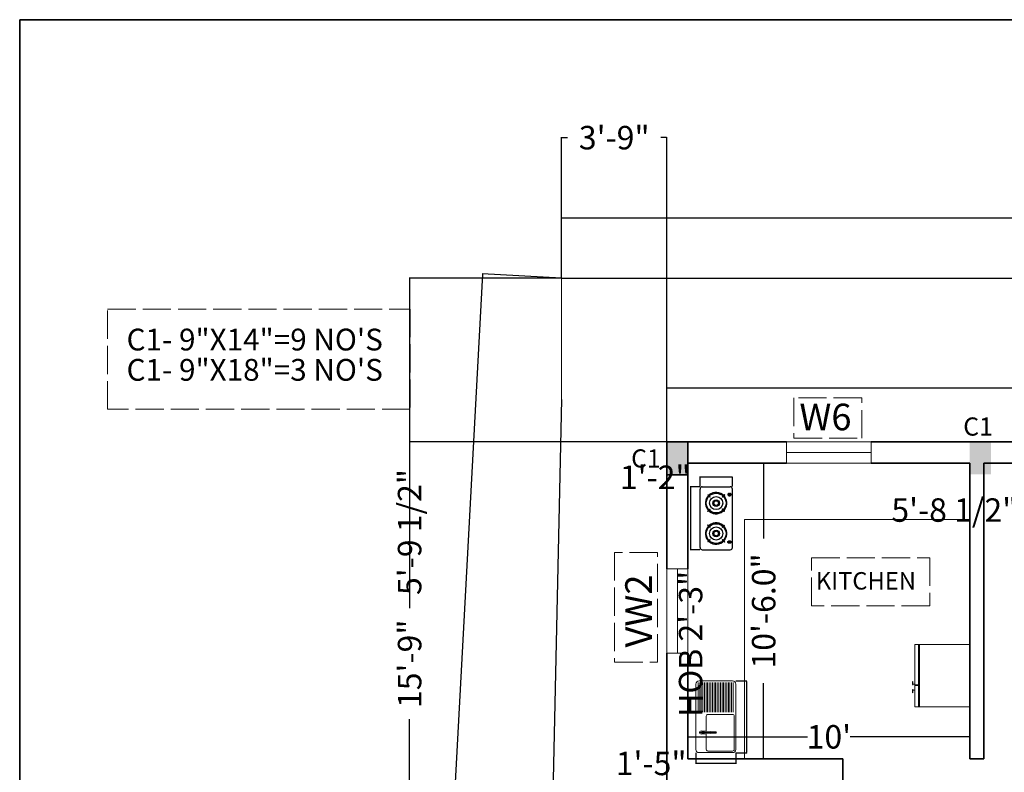
# Model space of a CAD drawing. Units: inches. Extents: x -269 to 4574, y -694 to 313.
# Tile 9 of 19: x -269 to 151, y -122 to 198. Entities that reach past the tile are written whole.
import ezdxf

# ---------------------------------------------------------------- set-up
doc = ezdxf.new("R2010")
doc.units = ezdxf.units.IN
doc.header["$MEASUREMENT"] = 0
doc.linetypes.add('ACAD_ISO02W100', pattern=[15, 12, -3])
for name, color, linetype, lineweight in [('A-ANNO-FRAM', 7, 'ACAD_ISO02W100', 13), ('A-ANNO-IDEN', 6, 'Continuous', 18), ('A-AREA-IDEN', 6, 'Continuous', 20), ('A-COLS', 5, 'Continuous', 35), ('A-COLS-IDEN', 6, 'Continuous', 18), ('A-COLS-PATT', 5, 'Continuous', 35), ('A-EQPM', 21, 'Continuous', 18), ('A-FLOR-CASE', 2, 'Continuous', 18), ('A-FLOR-FIXT', 21, 'Continuous', 18), ('BORDER', 7, 'Continuous', 35), ('C-PROP', 7, 'Continuous', 25), ('DIMENSION', 5, 'Continuous', 18), ('WALL', 1, 'Continuous', 35), ('WINDOWS', 2, 'Continuous', 18)]:
    doc.layers.add(name, color=color, linetype=linetype, lineweight=lineweight)
doc.layers.add('NOI THAT', color=42, linetype='Continuous')
doc.dimstyles.get("Standard").update_dxf_attribs({"dimtxt": 10, "dimasz": 0.18, "dimexe": 0.18, "dimexo": 0.0625, "dimgap": 0.09, "dimtad": 0, "dimdec": 1, "dimzin": 0, "dimdsep": 46, "dimlunit": 3, "dimtxsty": 'Standard', "dimcen": 0.09, "dimclrt": 7, "dimadec": 0, "dimazin": 0, "dimtfac": 1, "dimtdec": 1, "dimtofl": 0, "dimtmove": 0, "dimatfit": 3, "dimfxl": 1, "dimtolj": 1, "dimtzin": 0, "dimarcsym": 0})

# ---------------------------------------------------------------- blocks, each defined once
blk = doc.blocks.new('*D1')
at = {"layer": 'Defpoints', "color": 0, "lineweight": 0, "transparency": 16777216}
for p in [(451.14, 41.26), (7.14, 18.27), (451.14, 18.27)]:
    blk.add_point(p, dxfattribs=at)
at = {"layer": 'DIMENSION', "color": 0, "lineweight": -2, "transparency": 16777216}
for p, q in [((7.14, 18.33), (7.14, 41.44)), ((7.32, 41.26), (219.05, 41.26)), ((450.96, 41.26), (239.23, 41.26)), ((451.14, 18.33), (451.14, 41.44))]:
    blk.add_line(p, q, dxfattribs=at)
at = {"layer": 'DIMENSION', "color": 0, "lineweight": 0, "transparency": 16777216}
for points in [[(7.32, 41.29), (7.32, 41.23), (7.14, 41.26)], [(450.96, 41.29), (450.96, 41.23), (451.14, 41.26)]]:
    blk.add_solid(points, dxfattribs=at)
at = {"layer": 'DIMENSION', "color": 0, "transparency": 16777216, "insert": (229.14, 41.26), "char_height": 10, "attachment_point": 5}
blk.add_mtext("\\A1;37'", dxfattribs=at)
blk = doc.blocks.new('SINK90X50')
for p, q in [((-57, 553), (-430, 553)), ((-57, 533), (-430, 533)), ((-57, 513), (-430, 513)), ((192, 455), (177, 516)), ((187, 334), (177, 516)), ((197, 536), (197, 324)), ((202, 455), (217, 516)), ((207, 334), (217, 516)), ((-57, 493), (-430, 493)), ((-57, 473), (-430, 473)), ((-57, 453), (-430, 453)), ((-57, 433), (-430, 433)), ((-57, 413), (-430, 413)), ((-57, 393), (-430, 393)), ((-57, 373), (-430, 373)), ((-57, 353), (-430, 353)), ((-57, 333), (-430, 333)), ((-57, 313), (-430, 313)), ((-57, 293), (-430, 293)), ((-57, 273), (-430, 273)), ((-57, 253), (-430, 253)), ((-57, 233), (-430, 233)), ((-57, 213), (-430, 213)), ((-57, 193), (-430, 193)), ((-57, 173), (-430, 173)), ((-57, 153), (-430, 153)), ((-57, 133), (-430, 133)), ((-57, 113), (-430, 113))]:
    blk.add_line(p, q)
blk.add_lwpolyline([(450, 540, 0.414214), (410, 580), (-410, 580, 0.414214), (-450, 540), (-450, 120, 0.414214), (-410, 80), (410, 80, 0.414214), (450, 120)], format="xyb", close=True)
blk.add_lwpolyline([(181, 450), (-10, 450, 0.414214), (-30, 430), (-30, 120, 0.414214), (-10, 100), (410, 100, 0.414214), (430, 120), (430, 430, 0.414214), (410, 450), (214, 450)], format="xyb")
for centre, radius, start, end in [((197, 516), 20, 351.3062, 188.6938), ((197, 455), 5, 180, 0), ((197, 334), 10, 180, 0)]:
    blk.add_arc(centre, radius, start, end)
for points in [[(187, 506), (181, 513), (189, 496), (197, 479)], [(207, 506), (214, 513), (206, 496), (197, 479)]]:
    blk.add_open_spline(points, degree=3)
blk = doc.blocks.new('A$C2C6C0730')
at = {"layer": 'NOI THAT'}
for p, q in [((0, 1353), (0, 50)), ((670, 1403), (50, 1403)), ((720, 1353), (720, 50)), ((670, 0), (50, 0))]:
    blk.add_line(p, q, dxfattribs=at)
for points in [[(66, 1257, -0.070182), (81, 1254, -0.081942), (93, 1249, -0.106897), (102, 1239, -0.135195), (105, 1230, -0.135195), (102, 1220, -0.106897), (93, 1210, -0.081942), (81, 1205, -0.070182), (66, 1203, -0.070182), (50, 1205, -0.081942), (38, 1210, -0.106897), (30, 1220, -0.135195), (27, 1230, -0.135195), (30, 1239, -0.106897), (38, 1249, -0.081942), (50, 1254, -0.070182)], [(66, 146, 0.070182), (81, 148, 0.081942), (93, 154, 0.106897), (102, 163, 0.135195), (105, 173, 0.135195), (102, 183, 0.106897), (93, 192, 0.081942), (81, 198, 0.070182), (66, 200, 0.070182), (50, 198, 0.081942), (38, 192, 0.106897), (30, 183, 0.135195), (27, 173, 0.135195), (30, 163, 0.106897), (38, 154, 0.081942), (50, 148, 0.070182)]]:
    blk.add_lwpolyline(points, format="xyb", close=True, dxfattribs=at)
for points in [[(68, 1203), (68, 1257), (62, 1257), (62, 1203)], [(220, 1175), (171, 1223), (179, 1230), (227, 1182)], [(541, 1226), (493, 1177), (500, 1170), (548, 1219)], [(176, 861), (224, 909), (232, 902), (183, 853)], [(497, 897), (546, 849), (553, 856), (505, 904)], [(176, 542), (224, 494), (232, 501), (183, 550)], [(497, 506), (546, 554), (553, 547), (505, 498)], [(220, 228), (171, 180), (179, 172), (227, 221)], [(541, 177), (493, 225), (500, 233), (548, 184)], [(68, 200), (68, 146), (62, 146), (62, 200)]]:
    blk.add_lwpolyline(points, close=True, dxfattribs=at)
for centre, radius in [((362, 1040), 219), ((362, 1040), 145), ((362, 1040), 72.6), ((362, 1040), 51.5), ((362, 363), 219), ((362, 363), 145), ((362, 363), 72.6), ((362, 363), 51.5)]:
    blk.add_circle(centre, radius, dxfattribs=at)
for centre, radius, start, end in [((50, 1353), 50, 90, 180), ((670, 1353), 50, 0, 90), ((65, 1230), 19.4, 99.7177, 260.2823), ((65, 1230), 19.4, 279.9102, 80.0898), ((362, 1040), 238, 152.4796, 149.9329), ((362, 363), 238, 210.0671, 207.5204), ((50, 50), 50, 180, 270), ((65, 173), 19.4, 99.7177, 260.2823), ((65, 173), 19.4, 279.9102, 80.0898), ((670, 50), 50, 270, 0)]:
    blk.add_arc(centre, radius, start, end, dxfattribs=at)
blk = doc.blocks.new('*D16')
at = {"layer": 'Defpoints', "color": 0, "lineweight": 0, "transparency": 16777216}
for p in [(16.14, -107.35), (16.14, -116.73), (136.14, -116.73)]:
    blk.add_point(p, dxfattribs=at)
at = {"layer": 'DIMENSION', "color": 0, "lineweight": -2, "transparency": 16777216}
for p, q in [((16.14, -116.67), (16.14, -107.17)), ((16.32, -107.35), (67, -107.35)), ((135.96, -107.35), (85.27, -107.35)), ((136.14, -116.67), (136.14, -107.17))]:
    blk.add_line(p, q, dxfattribs=at)
at = {"layer": 'DIMENSION', "color": 0, "lineweight": 0, "transparency": 16777216}
for points in [[(16.32, -107.32), (16.32, -107.38), (16.14, -107.35)], [(135.96, -107.32), (135.96, -107.38), (136.14, -107.35)]]:
    blk.add_solid(points, dxfattribs=at)
at = {"layer": 'DIMENSION', "color": 0, "transparency": 16777216, "insert": (76.14, -107.35), "char_height": 10, "attachment_point": 5}
blk.add_mtext("\\A1;10'", dxfattribs=at)
blk = doc.blocks.new('*D17')
at = {"layer": 'Defpoints', "color": 0, "lineweight": 0, "transparency": 16777216}
for p in [(40.14, 9.27), (48.37, 9.27), (40.14, -116.73)]:
    blk.add_point(p, dxfattribs=at)
at = {"layer": 'DIMENSION', "color": 0, "lineweight": -2, "transparency": 16777216}
for p, q in [((40.2, 9.27), (48.55, 9.27)), ((48.37, 9.09), (48.37, -22.93)), ((48.37, -116.55), (48.37, -84.54)), ((40.2, -116.73), (48.55, -116.73))]:
    blk.add_line(p, q, dxfattribs=at)
at = {"layer": 'DIMENSION', "color": 0, "lineweight": 0, "transparency": 16777216}
for points in [[(48.34, 9.09), (48.4, 9.09), (48.37, 9.27)], [(48.34, -116.55), (48.4, -116.55), (48.37, -116.73)]]:
    blk.add_solid(points, dxfattribs=at)
at = {"layer": 'DIMENSION', "color": 0, "transparency": 16777216, "insert": (48.37, -53.73), "char_height": 10, "attachment_point": 5, "rotation": 90}
blk.add_mtext('\\A1;10\'-6.0"', dxfattribs=at)
blk = doc.blocks.new('*D32')
at = {"layer": 'Defpoints', "color": 0, "lineweight": 0, "transparency": 16777216}
for p in [(-37.71, 113.85), (478.29, 113.67), (478.29, 113.64)]:
    blk.add_point(p, dxfattribs=at)
at = {"layer": 'DIMENSION', "color": 0, "lineweight": -2, "transparency": 16777216}
for p, q in [((-37.71, 113.79), (-37.71, 113.46)), ((-37.53, 113.64), (210.2, 113.64)), ((478.11, 113.64), (230.38, 113.64)), ((478.29, 113.61), (478.29, 113.46))]:
    blk.add_line(p, q, dxfattribs=at)
at = {"layer": 'DIMENSION', "color": 0, "lineweight": 0, "transparency": 16777216}
for points in [[(-37.53, 113.67), (-37.53, 113.61), (-37.71, 113.64)], [(478.11, 113.67), (478.11, 113.61), (478.29, 113.64)]]:
    blk.add_solid(points, dxfattribs=at)
at = {"layer": 'DIMENSION', "color": 0, "transparency": 16777216, "insert": (220.29, 113.64), "char_height": 10, "attachment_point": 5}
blk.add_mtext("\\A1;43'", dxfattribs=at)
blk = doc.blocks.new('*D34')
at = {"layer": 'Defpoints', "color": 0, "lineweight": 0, "transparency": 16777216}
for p in [(-37.71, 88), (-102.08, -478.85), (-68.45, -480.67)]:
    blk.add_point(p, dxfattribs=at)
at = {"layer": 'DIMENSION', "color": 0, "lineweight": -2, "transparency": 16777216}
for p, q in [((-71.35, 89.64), (-85, -162.81)), ((-37.77, 88), (-71.52, 89.83)), ((-102.07, -478.67), (-88.43, -226.23)), ((-68.51, -480.67), (-102.26, -478.84))]:
    blk.add_line(p, q, dxfattribs=at)
at = {"layer": 'DIMENSION', "color": 0, "lineweight": 0, "transparency": 16777216}
for points in [[(-71.38, 89.64), (-71.32, 89.64), (-71.34, 89.82)], [(-102.1, -478.67), (-102.04, -478.67), (-102.08, -478.85)]]:
    blk.add_solid(points, dxfattribs=at)
at = {"layer": 'DIMENSION', "color": 0, "transparency": 16777216, "insert": (-86.71, -194.52), "char_height": 10, "attachment_point": 5, "rotation": 86.9054}
blk.add_mtext('\\A1;47\'-5.5"', dxfattribs=at)
blk = doc.blocks.new('GLAZ-36IN')
blk.add_line((0, 4.5), (36, 4.5))
blk.add_lwpolyline([(0, 9), (36, 9), (36, 0), (0, 0)], close=True)
blk = doc.blocks.new('COLUMN-9x14-PLAN')
h = blk.add_hatch(color=256)
h.dxf.hatch_style = 1
h.paths.add_polyline_path([(9, 14), (0, 14), (0, 0), (9, 0), (9, 5)])
blk = doc.blocks.new('*D61')
at = {"layer": 'Defpoints', "color": 0, "lineweight": 0, "transparency": 16777216}
for p in [(36.5, -83.55), (36.5, -114.1), (41.08, -114.1)]:
    blk.add_point(p, dxfattribs=at)
at = {"layer": 'DIMENSION', "color": 0, "lineweight": -2, "transparency": 16777216}
for p, q in [((36.56, -83.55), (41.26, -83.55)), ((41.08, -83.73), (41.08, -113.92)), ((36.56, -114.1), (41.26, -114.1)), ((41.08, -114.1), (41.08, -114.28))]:
    blk.add_line(p, q, dxfattribs=at)
at = {"layer": 'DIMENSION', "color": 0, "lineweight": 0, "transparency": 16777216}
for points in [[(41.05, -83.73), (41.11, -83.73), (41.08, -83.55)], [(41.05, -113.92), (41.11, -113.92), (41.08, -114.1)]]:
    blk.add_solid(points, dxfattribs=at)
at = {"layer": 'DIMENSION', "color": 7, "transparency": 16777216, "insert": (41.08, -173.89), "char_height": 10, "attachment_point": 5, "rotation": 90}
blk.add_mtext('\\A1;SINK 2\'-6 1/2"', dxfattribs=at)
blk = doc.blocks.new('*D62')
at = {"layer": 'Defpoints', "color": 0, "lineweight": 0, "transparency": 16777216}
for p in [(19.53, -114.1), (36.5, -114.1), (19.53, -118.68)]:
    blk.add_point(p, dxfattribs=at)
at = {"layer": 'DIMENSION', "color": 0, "lineweight": -2, "transparency": 16777216}
for p, q in [((19.53, -114.16), (19.53, -118.86)), ((36.5, -114.16), (36.5, -118.86)), ((19.53, -118.68), (19.35, -118.68)), ((36.32, -118.68), (19.71, -118.68))]:
    blk.add_line(p, q, dxfattribs=at)
at = {"layer": 'DIMENSION', "color": 0, "lineweight": 0, "transparency": 16777216}
for points in [[(19.71, -118.65), (19.71, -118.71), (19.53, -118.68)], [(36.32, -118.65), (36.32, -118.71), (36.5, -118.68)]]:
    blk.add_solid(points, dxfattribs=at)
at = {"layer": 'DIMENSION', "color": 7, "transparency": 16777216, "insert": (0.45, -118.68), "char_height": 10, "attachment_point": 5}
blk.add_mtext('\\A1;1\'-5"', dxfattribs=at)
blk = doc.blocks.new('*D63')
at = {"layer": 'Defpoints', "color": 0, "lineweight": 0, "transparency": 16777216}
for p in [(21.28, -0.84), (17.25, -27.7), (21.28, -27.7)]:
    blk.add_point(p, dxfattribs=at)
at = {"layer": 'DIMENSION', "color": 0, "lineweight": -2, "transparency": 16777216}
for p, q in [((21.22, -0.84), (17.07, -0.84)), ((17.25, -1.02), (17.25, -27.52)), ((21.22, -27.7), (17.07, -27.7)), ((17.25, -27.7), (17.25, -27.88))]:
    blk.add_line(p, q, dxfattribs=at)
at = {"layer": 'DIMENSION', "color": 0, "lineweight": 0, "transparency": 16777216}
for points in [[(17.22, -1.02), (17.28, -1.02), (17.25, -0.84)], [(17.22, -27.52), (17.28, -27.52), (17.25, -27.7)]]:
    blk.add_solid(points, dxfattribs=at)
at = {"layer": 'DIMENSION', "color": 7, "transparency": 16777216, "insert": (17.25, -67.74), "char_height": 10, "attachment_point": 5, "rotation": 90}
blk.add_mtext('\\A1;HOB 2\'-3"', dxfattribs=at)
blk = doc.blocks.new('*D64')
at = {"layer": 'Defpoints', "color": 0, "lineweight": 0, "transparency": 16777216}
for p in [(21.28, 3.19), (21.28, -0.84), (35.07, -0.84)]:
    blk.add_point(p, dxfattribs=at)
at = {"layer": 'DIMENSION', "color": 0, "lineweight": -2, "transparency": 16777216}
for p, q in [((21.28, 3.19), (21.1, 3.19)), ((21.28, -0.78), (21.28, 3.37)), ((34.89, 3.19), (21.46, 3.19)), ((35.07, -0.78), (35.07, 3.37))]:
    blk.add_line(p, q, dxfattribs=at)
at = {"layer": 'DIMENSION', "color": 0, "lineweight": 0, "transparency": 16777216}
for points in [[(21.46, 3.22), (21.46, 3.16), (21.28, 3.19)], [(34.89, 3.22), (34.89, 3.16), (35.07, 3.19)]]:
    blk.add_solid(points, dxfattribs=at)
at = {"layer": 'DIMENSION', "color": 7, "transparency": 16777216, "insert": (2.2, 3.19), "char_height": 10, "attachment_point": 5}
blk.add_mtext('\\A1;1\'-2"', dxfattribs=at)
blk = doc.blocks.new('*D66')
at = {"layer": 'Defpoints', "color": 0, "lineweight": 0, "transparency": 16777216}
for p in [(167.97, -10.77), (167.97, -24.12), (236.53, -24.12)]:
    blk.add_point(p, dxfattribs=at)
at = {"layer": 'DIMENSION', "color": 0, "lineweight": -2, "transparency": 16777216}
for p, q in [((167.97, -10.77), (167.79, -10.77)), ((167.97, -24.05), (167.97, -10.59)), ((236.35, -10.77), (168.15, -10.77)), ((236.53, -24.05), (236.53, -10.59))]:
    blk.add_line(p, q, dxfattribs=at)
at = {"layer": 'DIMENSION', "color": 0, "lineweight": 0, "transparency": 16777216}
for points in [[(168.15, -10.74), (168.15, -10.8), (167.97, -10.77)], [(236.35, -10.74), (236.35, -10.8), (236.53, -10.77)]]:
    blk.add_solid(points, dxfattribs=at)
at = {"layer": 'DIMENSION', "color": 7, "transparency": 16777216, "insert": (129.6, -10.77), "char_height": 10, "attachment_point": 5}
blk.add_mtext('\\A1;5\'-8 1/2"', dxfattribs=at)
blk = doc.blocks.new('*D74')
at = {"layer": 'Defpoints', "color": 0, "lineweight": 0, "transparency": 16777216}
for p in [(-37.71, 88), (-102.45, 18.27), (7.14, 18.27)]:
    blk.add_point(p, dxfattribs=at)
at = {"layer": 'DIMENSION', "color": 0, "lineweight": -2, "transparency": 16777216}
for p, q in [((-37.77, 88), (-102.63, 88)), ((-102.45, 87.82), (-102.45, 18.45)), ((7.07, 18.27), (-102.63, 18.27)), ((-102.45, 18.27), (-102.45, 18.09))]:
    blk.add_line(p, q, dxfattribs=at)
at = {"layer": 'DIMENSION', "color": 0, "lineweight": 0, "transparency": 16777216}
for points in [[(-102.48, 87.82), (-102.42, 87.82), (-102.45, 88)], [(-102.48, 18.45), (-102.42, 18.45), (-102.45, 18.27)]]:
    blk.add_solid(points, dxfattribs=at)
at = {"layer": 'DIMENSION', "color": 7, "transparency": 16777216, "insert": (-102.45, -20.1), "char_height": 10, "attachment_point": 5, "rotation": 90}
blk.add_mtext('\\A1;5\'-9 1/2"', dxfattribs=at)
blk = doc.blocks.new('*D75')
at = {"layer": 'Defpoints', "color": 0, "lineweight": 0, "transparency": 16777216}
for p in [(7.14, 147.85), (-37.71, 88), (7.14, 18.27)]:
    blk.add_point(p, dxfattribs=at)
at = {"layer": 'DIMENSION', "color": 0, "lineweight": -2, "transparency": 16777216}
for p, q in [((-37.71, 88.06), (-37.71, 148.03)), ((-37.53, 147.85), (-35.14, 147.85)), ((6.96, 147.85), (4.57, 147.85)), ((7.14, 18.33), (7.14, 148.03))]:
    blk.add_line(p, q, dxfattribs=at)
at = {"layer": 'DIMENSION', "color": 0, "lineweight": 0, "transparency": 16777216}
for points in [[(-37.53, 147.88), (-37.53, 147.82), (-37.71, 147.85)], [(6.96, 147.88), (6.96, 147.82), (7.14, 147.85)]]:
    blk.add_solid(points, dxfattribs=at)
at = {"layer": 'DIMENSION', "color": 7, "transparency": 16777216, "insert": (-15.28, 147.85), "char_height": 10, "attachment_point": 5}
blk.add_mtext('\\A1;3\'-9"', dxfattribs=at)
blk = doc.blocks.new('*D76')
at = {"layer": 'Defpoints', "color": 0, "lineweight": 0, "transparency": 16777216}
for p in [(7.14, 18.27), (-102.45, -170.73), (16.14, -170.73)]:
    blk.add_point(p, dxfattribs=at)
at = {"layer": 'DIMENSION', "color": 0, "lineweight": -2, "transparency": 16777216}
for p, q in [((7.07, 18.27), (-102.63, 18.27)), ((-102.45, 18.09), (-102.45, -52.57)), ((-102.45, -170.55), (-102.45, -99.89)), ((16.07, -170.73), (-102.63, -170.73))]:
    blk.add_line(p, q, dxfattribs=at)
at = {"layer": 'DIMENSION', "color": 0, "lineweight": 0, "transparency": 16777216}
for points in [[(-102.48, 18.09), (-102.42, 18.09), (-102.45, 18.27)], [(-102.48, -170.55), (-102.42, -170.55), (-102.45, -170.73)]]:
    blk.add_solid(points, dxfattribs=at)
at = {"layer": 'DIMENSION', "color": 7, "transparency": 16777216, "insert": (-102.45, -76.23), "char_height": 10, "attachment_point": 5, "rotation": 90}
blk.add_mtext('\\A1;15\'-9"', dxfattribs=at)

msp = doc.modelspace()

# ---------------------------------------------------------------- hatches: boundary and pattern name
at = {"layer": 'A-COLS-PATT'}
h = msp.add_hatch(color=256, dxfattribs=at)
h.dxf.hatch_style = 1
h.paths.add_polyline_path([(16.14, 18.27), (7.14, 18.27), (7.14, 4.27), (16.14, 4.27), (16.14, 9.27)])

# ---------------------------------------------------------------- linework, layer by layer
at = {"layer": 'A-ANNO-FRAM'}
for points in [[(-231.08, 74.85), (-102.18, 74.85), (-102.18, 32.18), (-231.08, 32.18)], [(90.18, 36.98), (61.24, 36.98), (61.24, 19.84), (90.18, 19.84)], [(3.2, -28.82), (-15.16, -28.82), (-15.16, -75.62), (3.2, -75.62)], [(68.75, -31.06), (119.14, -31.06), (119.14, -51.51), (68.75, -51.51)]]:
    msp.add_lwpolyline(points, close=True, dxfattribs=at)
at = {"layer": 'A-COLS'}
for p, q in [((16.14, 9.27), (16.14, 18.27)), ((7.14, 4.27), (16.14, 4.27))]:
    msp.add_line(p, q, dxfattribs=at)
at = {"layer": 'A-EQPM'}
for points, invisible_edges in [([(112.8, -85.17, 51.35), (112.8, -85.17, 51.35), (112.8, -68.06, 3.11), (112.8, -85.17, 3.11)], 2), ([(112.8, -68.06, 3.11), (112.8, -68.06, 3.11), (112.8, -85.17, 51.35), (112.8, -68.06, 51.35)], 2), ([(114.35, -68.06, 3.11), (114.35, -68.06, 3.11), (112.8, -68.06, 51.35), (114.35, -68.06, 51.35)], 2), ([(112.8, -68.06, 51.35), (112.8, -68.06, 51.35), (114.35, -68.06, 3.11), (112.8, -68.06, 3.11)], 2), ([(112.8, -68.06, 51.35), (112.8, -68.06, 51.35), (114.35, -85.17, 51.35), (114.35, -68.06, 51.35)], 2), ([(114.35, -85.17, 51.35), (114.35, -85.17, 51.35), (112.8, -68.06, 51.35), (112.8, -85.17, 51.35)], 2), ([(114.74, -68.06), (114.74, -68.06), (136.14, -68.06, 51.35), (136.14, -68.06)], 2), ([(136.14, -68.06, 51.35), (136.14, -68.06, 51.35), (114.74, -68.06), (114.74, -68.06, 51.35)], 2), ([(114.74, -94.51, 3.11), (114.74, -94.51, 3.11), (114.74, -68.06), (114.74, -94.51)], 2), ([(114.74, -68.06), (114.74, -68.06), (114.74, -94.51, 3.11), (114.74, -68.06, 3.11)], 2), ([(114.74, -68.06, 51.35), (114.74, -68.06, 51.35), (136.14, -94.51, 51.35), (136.14, -68.06, 51.35)], 2), ([(136.14, -94.51, 51.35), (136.14, -94.51, 51.35), (114.74, -68.06, 51.35), (114.74, -94.51, 51.35)], 2), ([(136.14, -68.06, 51.35), (136.14, -68.06, 51.35), (136.14, -94.51), (136.14, -68.06)], 2), ([(136.14, -94.51), (136.14, -94.51), (136.14, -68.06, 51.35), (136.14, -94.51, 51.35)], 2), ([(112.8, -94.51, 51.35), (112.8, -94.51, 51.35), (112.8, -85.56, 3.11), (112.8, -94.51, 3.11)], 2), ([(112.8, -85.56, 3.11), (112.8, -85.56, 3.11), (112.8, -94.51, 51.35), (112.8, -85.56, 51.35)], 2), ([(114.35, -85.56, 51.35), (114.35, -85.56, 51.35), (112.8, -94.51, 51.35), (114.35, -94.51, 51.35)], 2), ([(112.8, -94.51, 51.35), (112.8, -94.51, 51.35), (114.35, -85.56, 51.35), (112.8, -85.56, 51.35)], 2), ([(114.35, -94.51, 3.11), (114.35, -94.51, 3.11), (114.35, -94.51, 51.35), (112.8, -94.51, 51.35)], 9), ([(112.8, -94.51, 51.35), (112.8, -94.51, 51.35), (112.8, -94.51, 3.11), (114.35, -94.51, 3.11)], 9), ([(114.74, -94.51), (114.74, -94.51), (136.14, -94.51), (136.14, -94.51, 51.35)], 9), ([(136.14, -94.51, 51.35), (136.14, -94.51, 51.35), (114.74, -94.51, 51.35), (114.74, -94.51)], 9)]:
    msp.add_3dface(points, dxfattribs=dict(at, invisible_edges=invisible_edges))
at = {"layer": 'A-FLOR-CASE'}
for p, q in [((40.14, -116.73), (40.14, -14.73)), ((40.14, -14.73), (136.14, -14.73))]:
    msp.add_line(p, q, dxfattribs=at)
at = {"layer": 'BORDER'}
msp.add_lwpolyline([(-268.51, 198.09), (666.62, 198.09), (666.62, -693.82), (-268.51, -693.82)], close=True, dxfattribs=at)
at = {"layer": 'C-PROP'}
for p, q in [((-37.71, 88), (478.29, 88)), ((-37.71, 36.26), (-49.71, -506.83))]:
    msp.add_line(p, q, dxfattribs=at)
at = {"layer": 'DIMENSION'}
msp.add_line((-37.71, 36.32), (-37.71, 113.85), dxfattribs=at)
msp.add_solid([(-37.53, 113.7), (-37.53, 113.64), (-37.71, 113.67)], dxfattribs=at)
at = {"layer": 'WALL'}
for p, q in [((7.14, 18.27), (58.14, 18.27)), ((7.14, -35.73), (7.14, 18.27)), ((94.14, 18.27), (181.14, 18.27)), ((16.14, 9.27), (58.14, 9.27)), ((16.14, -35.73), (16.14, 9.27)), ((94.14, 9.27), (136.14, 9.27)), ((136.14, -116.73), (136.14, 9.27)), ((142.14, 9.27), (181.14, 9.27)), ((142.14, -116.73), (142.14, 9.27)), ((7.14, -134.73), (7.14, -71.73)), ((16.14, -116.73), (16.14, -71.73)), ((16.14, -116.73), (82.14, -116.73)), ((82.14, -144.99), (82.14, -116.73)), ((136.14, -116.73), (142.14, -116.73))]:
    msp.add_line(p, q, dxfattribs=at)

# ---------------------------------------------------------------- block references
at = {"layer": 'A-COLS'}
msp.add_blockref('COLUMN-9x14-PLAN', (136.14, 4.44), dxfattribs=at)
at = {"layer": 'A-EQPM', "xscale": 0.0191519776240158, "yscale": 0.0191519776240158, "zscale": 0.0191519776240158, "rotation": 180}
msp.add_blockref('A$C2C6C0730', (35.07, -0.84), dxfattribs=at)
at = {"layer": 'A-FLOR-FIXT', "xscale": 0.0339358373266139, "yscale": -0.0339358373266139, "zscale": 0.0339358373266139, "rotation": 270}
msp.add_blockref('SINK90X50', (39.21, -98.82), dxfattribs=at)
at = {"layer": 'WINDOWS'}
msp.add_blockref('GLAZ-36IN', (58.14, 9.27), dxfattribs=at)
at = {"layer": 'WINDOWS', "extrusion": (0, 0, -1), "zscale": -1, "rotation": 270}
msp.add_blockref('GLAZ-36IN', (-16.14, -35.73), dxfattribs=at)

# ---------------------------------------------------------------- texts
at = {"layer": 'A-ANNO-IDEN'}
msp.add_text('W6', height=11.343, dxfattribs=at).set_placement((63.6, 23.21))
msp.add_text('VW2', height=11.343, rotation=90, dxfattribs=at).set_placement((0.75, -69.31))
at = {"layer": 'A-AREA-IDEN'}
msp.add_text('KITCHEN ', height=7.418, dxfattribs=at).set_placement((70.57, -44.62))
at = {"layer": 'A-COLS-IDEN'}
for s, height, p in [('C1- 9"X14"=9 NO\'S', 9.2792, (-222.98, 57.21)), ('C1- 9"X18"=3 NO\'S', 9.2792, (-222.98, 44.31)), ('C1', 7.741, (133.38, 20.94)), ('C1', 7.741, (-8.08, 7.35))]:
    msp.add_text(s, height=height, dxfattribs=at).set_placement(p)

# ---------------------------------------------------------------- dimensions: what is measured, and where the dimension line sits
at = {"layer": 'DIMENSION'}
for base, p1, p2, override, picture, middle in [((7.137, 147.8534), (-37.7055, 87.9997), (7.137, 18.2683), {"dimdec": 1, "dimlfac": 1, "dimrnd": 0, "dimzin": 1, "dimdsep": 46, "dimlunit": 4, "dimfrac": 2}, '*D75', (-15.2842, 147.8534)), ((478.29, 113.64), (-37.71, 113.85), (478.29, 113.67), {"dimclrd": 0, "dimclre": 0, "dimclrt": 0}, '*D32', (220.29, 113.64)), ((451.14, 41.26), (7.14, 18.27), (451.14, 18.27), {"dimclrd": 0, "dimclre": 0, "dimclrt": 0}, '*D1', (229.14, 41.26)), ((16.14, -107.35), (136.14, -116.73), (16.14, -116.73), {"dimclrd": 0, "dimclre": 0, "dimclrt": 0}, '*D16', (76.14, -107.35))]:
    dim = msp.add_linear_dim(base=base, p1=p1, p2=p2, dimstyle='Standard', override=override, dxfattribs=at)
    dim.commit()
    dim.dimension.update_dxf_attribs({"geometry": picture, "text_midpoint": middle})
dim = msp.add_aligned_dim(p1=(-37.71, 88), p2=(-68.45, -480.67), distance=-33.68, dimstyle='Standard', override={"dimclrd": 0, "dimclre": 0, "dimclrt": 0}, dxfattribs=at)
dim.commit()
dim.dimension.update_dxf_attribs({"geometry": '*D34', "text_midpoint": (-86.71, -194.52)})
for base, p1, p2, angle, override, picture, middle in [((-102.45, 18.27), (-37.71, 88), (7.14, 18.27), 90, {"dimdec": 1, "dimlfac": 1, "dimrnd": 0, "dimzin": 1, "dimdsep": 46, "dimlunit": 4, "dimfrac": 2}, '*D74', (-102.45, -20.1)), ((-102.45, -170.73), (7.14, 18.27), (16.14, -170.73), 90, {"dimdec": 1, "dimlfac": 1, "dimrnd": 0, "dimzin": 1, "dimdsep": 46, "dimlunit": 4, "dimfrac": 2}, '*D76', (-102.45, -76.23)), ((21.28, 3.19), (35.07, -0.84), (21.28, -0.84), 180, {"dimdec": 1, "dimlfac": 1, "dimrnd": 0, "dimzin": 1, "dimdsep": 46, "dimlunit": 4, "dimfrac": 2}, '*D64', (2.2, 3.19)), ((48.37, 9.27), (40.14, -116.73), (40.14, 9.27), 90, {"dimclrd": 0, "dimclre": 0, "dimclrt": 0}, '*D17', (48.37, -53.73)), ((167.97, -10.77), (236.53, -24.12), (167.97, -24.12), 180, {"dimdec": 1, "dimlfac": 1, "dimrnd": 0, "dimzin": 1, "dimdsep": 46, "dimlunit": 4, "dimfrac": 2}, '*D66', (129.6, -10.77)), ((19.53, -118.68), (36.5, -114.1), (19.53, -114.1), 180, {"dimdec": 1, "dimlfac": 1, "dimrnd": 0, "dimzin": 1, "dimdsep": 46, "dimlunit": 4, "dimfrac": 2}, '*D62', (0.45, -118.68))]:
    dim = msp.add_linear_dim(base=base, p1=p1, p2=p2, angle=angle, dimstyle='Standard', override=override, dxfattribs=at)
    dim.commit()
    dim.dimension.update_dxf_attribs({"geometry": picture, "text_midpoint": middle})
for base, p1, p2, text, picture, middle in [((17.25, -27.7), (21.28, -0.84), (21.28, -27.7), 'HOB <>', '*D63', (17.25, -67.74)), ((41.0773, -114.0959), (36.496, -83.5537), (36.496, -114.0959), 'SINK <>', '*D61', (41.0773, -173.8897))]:
    dim = msp.add_linear_dim(base=base, p1=p1, p2=p2, angle=270, text=text, dimstyle='Standard', override={"dimdec": 1, "dimlfac": 1, "dimrnd": 0, "dimzin": 1, "dimdsep": 46, "dimlunit": 4, "dimfrac": 2}, dxfattribs=at)
    dim.commit()
    dim.dimension.update_dxf_attribs({"geometry": picture, "text_midpoint": middle})

# ---------------------------------------------------------------- meshes
at = {"layer": 'A-EQPM'}
mesh = msp.add_polyface(dxfattribs=at)
corners = [(112.8, -85.17, 51.35), (112.8, -85.56, 51.35), (112.8, -85.56, 3.11), (112.8, -85.17, 3.11), (114.35, -85.17, 51.35), (114.35, -85.56, 51.35), (114.74, -68.06, 51.35), (114.35, -68.06, 51.35), (114.35, -68.06, 3.11), (114.74, -68.06, 3.11), (114.74, -94.51, 51.35), (114.35, -94.51, 51.35), (114.74, -94.51, 3.11), (114.35, -94.51, 3.11)]
mesh.append_faces([[corners[k] for k in face] for face in [(0, 5, 4), (5, 0, 1), (6, 11, 10), (11, 6, 7)]], dxfattribs={"vtx0": -1})
mesh.append_faces([[corners[k] for k in face] for face in [(2, 1, 0), (0, 3, 2), (8, 7, 6), (6, 9, 8), (11, 13, 12), (12, 10, 11)]], dxfattribs={"vtx2": -1})
mesh = msp.add_polyface(dxfattribs=at)
corners = [(111.97, -85.38, 24.76), (111.97, -83.73, 24.76), (111.97, -83.73, 39.6), (111.97, -85.38, 39.6), (111.79, -84.99, 24.76), (111.79, -84.99, 39.6), (111.78, -84.63, 24.76), (111.78, -84.63, 39.6), (111.78, -84.22, 24.76), (111.78, -84.22, 39.6), (111.82, -83.9, 24.76), (111.82, -83.9, 39.6), (111.97, -88.68, 24.76), (111.97, -87.03, 24.76), (111.97, -88.68, 39.6), (111.97, -87.03, 39.6), (111.79, -87.42, 24.76), (111.79, -87.42, 39.6), (111.78, -87.78, 24.76), (111.78, -87.78, 39.6), (111.78, -88.18, 24.76), (111.78, -88.18, 39.6), (111.82, -88.5, 24.76), (111.82, -88.5, 39.6), (112.8, -87.44, 39.6), (111.97, -87.44, 39.6), (112.8, -87.44, 24.76), (111.97, -87.44, 24.76), (112.8, -84.97, 39.6), (111.97, -84.97, 39.6), (112.8, -84.97, 24.76), (111.97, -84.97, 24.76)]
mesh.append_faces([[corners[k] for k in face] for face in [(2, 0, 3), (3, 4, 5), (5, 6, 7), (7, 8, 9), (9, 10, 11), (11, 1, 2), (14, 13, 12), (14, 13, 15), (15, 16, 13), (17, 18, 16), (19, 20, 18), (21, 22, 20), (23, 12, 22), (26, 25, 24), (25, 26, 27), (30, 29, 28), (29, 30, 31), (13, 14, 15), (14, 13, 12)]], dxfattribs={"vtx0": -1})
mesh.append_faces([[corners[k] for k in face] for face in [(2, 1, 0), (3, 0, 4), (5, 4, 6), (7, 6, 8), (9, 8, 10), (11, 10, 1), (15, 17, 16), (17, 19, 18), (19, 21, 20), (21, 23, 22), (23, 14, 12), (1, 2, 3), (3, 0, 1)]], dxfattribs={"vtx2": -1})

doc.saveas('drawing.dxf')
